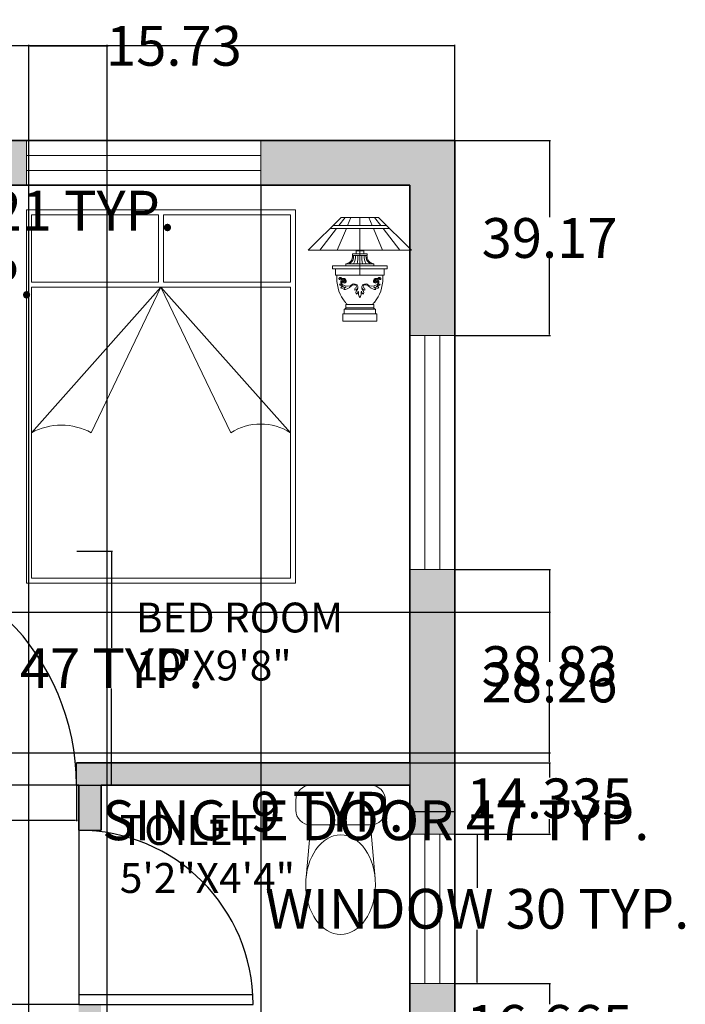
# Model space of a CAD drawing. Units: inches. Extents: x -24 to 368, y -370 to 58.
# Tile 9 of 9: x 235 to 368, y -140 to 58. Entities that reach past the tile are written whole.
import ezdxf

# ---------------------------------------------------------------- set-up
doc = ezdxf.new("R2010")
doc.units = ezdxf.units.IN
doc.header["$MEASUREMENT"] = 0
for name, color, linetype, lineweight in [('A-ANNO-DIMS', 2, 'Continuous', 18), ('A-AREA-IDEN', 7, 'Continuous', 18), ('A-FLOR-FIXT', 8, 'Continuous', 18), ('A-WALL', 7, 'Continuous', 35), ('Furniture', 7, 'Continuous', 15)]:
    doc.layers.add(name, color=color, linetype=linetype, lineweight=lineweight)
for name, color, linetype, lineweight, true_color in [('A-DOOR', 40, 'Continuous', 25, 0xf8d731), ('A-GLAZ', 30, 'Continuous', 18, 0xf26722), ('A-WALL-PATT', 18, 'Continuous', 13, 0x000000)]:
    doc.layers.add(name, color=color, linetype=linetype, lineweight=lineweight, true_color=true_color)
doc.styles.get("Standard").update_dxf_attribs({"font": 'arial.ttf'})
doc.dimstyles.get("Standard").update_dxf_attribs({"dimtxt": 8, "dimasz": 0.18, "dimexe": 0.18, "dimexo": 0.0625, "dimgap": 0.09, "dimtad": 0, "dimtih": 1, "dimtoh": 1, "dimdec": 4, "dimzin": 0, "dimdsep": 46, "dimlunit": 3, "dimtxsty": 'Standard', "dimcen": 0.09, "dimclre": 5, "dimclrt": 6, "dimadec": 0, "dimazin": 0, "dimtfac": 1, "dimtdec": 4, "dimtofl": 0, "dimtmove": 0, "dimatfit": 3, "dimfxl": 1, "dimtolj": 1, "dimtzin": 0, "dimarcsym": 0})

# ---------------------------------------------------------------- blocks, each defined once
blk = doc.blocks.new('LAMP-BEDSIDE')
for p, q in [((6.65, 20.8), (0, 14.26)), ((6.17, 19.19), (7.42, 20.8)), ((6.65, 20.8), (14.09, 20.8)), ((8.59, 20.8), (7.91, 19.19)), ((10.37, 20.8), (10.37, 19.19)), ((12.15, 20.8), (12.83, 19.19)), ((14.57, 19.19), (13.31, 20.8)), ((14.09, 20.8), (20.74, 14.26)), ((2.33, 14.26), (5.71, 18.6)), ((4.42, 18.6), (16.32, 18.6)), ((5.01, 19.19), (15.72, 19.19)), ((7.66, 18.6), (5.82, 14.26)), ((10.37, 18.6), (10.37, 9.21)), ((13.08, 18.6), (14.92, 14.26)), ((18.41, 14.26), (15.02, 18.6)), ((0, 14.26), (20.74, 14.26)), ((9.6, 14.09), (11.14, 14.09)), ((9.6, 14.09), (9.6, 13.52)), ((11.14, 14.09), (11.14, 13.52)), ((8.92, 13.52), (11.81, 13.52)), ((8.92, 13.52), (8.92, 13.19)), ((8.92, 13.19), (11.81, 13.19)), ((11.81, 13.52), (11.81, 13.19)), ((4.88, 11.13), (4.88, 10.49)), ((4.88, 11.13), (15.86, 11.13)), ((4.88, 10.49), (15.86, 10.49)), ((5.48, 10.49), (5.48, 9.21)), ((7.53, 11.52), (13.2, 11.52)), ((7.53, 11.52), (7.53, 11.13)), ((13.2, 11.52), (13.2, 11.13)), ((15.26, 10.49), (15.26, 9.21)), ((15.86, 11.13), (15.86, 10.49)), ((5.48, 9.21), (15.26, 9.21)), ((5.76, 9.21), (5.76, 8.59)), ((14.98, 9.21), (14.98, 8.59)), ((7.24, 2.43), (10.37, 2.43)), ((7.24, 2.43), (7.24, 1.48)), ((7.53, 3.34), (10.37, 3.34)), ((7.53, 3.34), (7.53, 2.65)), ((7.53, 2.65), (10.37, 2.65)), ((13.2, 3.34), (10.37, 3.34)), ((13.2, 2.65), (10.37, 2.65)), ((13.5, 2.43), (10.37, 2.43)), ((13.2, 3.34), (13.2, 2.65)), ((13.5, 2.43), (13.5, 1.48)), ((6.96, 1.48), (6.96, 0)), ((6.96, 1.48), (7.24, 1.48)), ((6.96, 0), (10.37, 0)), ((7.24, 1.48), (10.37, 1.48)), ((13.5, 1.48), (10.37, 1.48)), ((13.77, 0), (10.37, 0)), ((13.77, 1.48), (13.5, 1.48)), ((13.77, 1.48), (13.77, 0))]:
    blk.add_line(p, q)
for centre, radius, start, end in [((7.4, 13.04), 1.53, 274.9221, 5.4044), ((7.51, 13), 1.63, 295.0919, 6.6681), ((6.74, 12.97), 2.77, 328.5732, 4.5839), ((4.28, 12.92), 5.72, 345.8511, 2.7031), ((16.46, 12.92), 5.72, 177.2969, 194.1489), ((14, 12.97), 2.77, 175.4161, 211.4268), ((13.22, 13), 1.63, 173.3319, 244.9081), ((13.33, 13.04), 1.53, 174.5956, 265.0779), ((13.2, 8.5), 7.44, 179.3119, 219.4824), ((6.29, 8.51), 0.158, 124.9924, 335.335), ((6.45, 8.39), 0.355, 11.1092, 135.0155), ((6.39, 8.42), 0.0502, 145.048, 23.2806), ((6.51, 8.39), 0.171, 352.7452, 159.4145), ((7.39, 7.88), 0.87, 145.6908, 234.6789), ((7.4, 7.83), 0.668, 137.9008, 234.3868), ((7.12, 8.07), 0.5, 320.8911, 130.3323), ((7.11, 7.94), 0.236, 29.1955, 234.854), ((7.14, 8.08), 0.309, 326.7711, 139.3622), ((7.2, 8), 0.128, 26.7504, 223.4128), ((13.61, 8.07), 0.5, 49.6677, 219.1089), ((7.54, 8.5), 7.44, 320.5176, 0.6881), ((13.6, 8.08), 0.309, 40.6378, 213.2289), ((13.63, 7.94), 0.236, 305.146, 150.8045), ((13.54, 8), 0.128, 316.5872, 153.2496), ((13.34, 7.83), 0.668, 305.6132, 42.0992), ((13.34, 7.88), 0.87, 305.3211, 34.3092), ((14.29, 8.39), 0.355, 44.9845, 168.8908), ((14.23, 8.39), 0.171, 20.5855, 187.2548), ((14.45, 8.51), 0.158, 204.665, 55.0076), ((14.35, 8.42), 0.0502, 156.7194, 34.952), ((6.44, 6.9), 0.527, 30.7639, 106.5031), ((6.66, 7.53), 0.391, 199.4301, 258.0626), ((6.99, 6.45), 0.534, 81.7725, 150.3347), ((6.86, 7.15), 0.552, 231.7834, 300.6647), ((6.55, 6.3), 0.85, 53.0509, 88.4488), ((7.24, 8), 0.363, 223.4201, 318.9658), ((7.88, 8.48), 1.48, 232.7522, 313.7075), ((7.25, 8.05), 0.203, 224.103, 315.897), ((7.49, 6.32), 0.495, 75.8737, 133.8842), ((7.68, 6.3), 0.502, 98.3136, 177.606), ((7.04, 8.37), 2.05, 274.0547, 309.0162), ((5.53, 10.82), 4.92, 304.6293, 311.2979), ((9.22, 6.66), 0.644, 58.6818, 132.9572), ((9.12, 6.87), 0.587, 71.5671, 111.734), ((9.36, 6.81), 0.621, 342.0461, 94.8157), ((9.69, 6.38), 0.339, 108.5318, 204.8769), ((9.33, 6.92), 0.689, 273.9841, 333.6418), ((9.32, 6.94), 0.352, 316.7375, 49.0095), ((10.14, 5.79), 0.564, 138.2432, 224.6957), ((9.31, 6.66), 0.643, 310.3655, 356.3809), ((8.93, 6.11), 1.09, 318.697, 356.3018), ((9.3, 5.7), 0.788, 353.0671, 25.9825), ((11.43, 5.7), 0.788, 154.0175, 186.9329), ((11.81, 6.11), 1.09, 183.6982, 221.303), ((11.38, 6.81), 0.621, 85.1843, 197.9539), ((11.41, 6.92), 0.689, 206.3582, 266.0159), ((11.43, 6.66), 0.643, 183.6191, 229.6345), ((10.59, 5.79), 0.564, 315.3043, 41.7568), ((11.41, 6.94), 0.352, 130.9905, 223.2625), ((11.05, 6.38), 0.339, 335.1231, 71.4682), ((11.52, 6.66), 0.644, 47.0428, 121.3182), ((11.62, 6.87), 0.587, 68.266, 108.4329), ((12.85, 8.48), 1.48, 226.2925, 307.2478), ((15.2, 10.82), 4.92, 228.7021, 235.3707), ((13.7, 8.37), 2.05, 230.9838, 265.9453), ((13.25, 6.32), 0.495, 46.1158, 104.1263), ((13.05, 6.3), 0.502, 2.394, 81.6864), ((13.5, 8), 0.363, 221.0342, 316.5799), ((13.48, 8.05), 0.203, 224.103, 315.897), ((13.87, 7.15), 0.552, 239.3353, 308.2166), ((14.18, 6.3), 0.85, 91.5512, 126.9491), ((13.75, 6.45), 0.534, 29.6653, 98.2275), ((14.3, 6.9), 0.527, 73.4969, 149.2361), ((14.08, 7.53), 0.391, 281.9374, 340.5699), ((12.16, 5.83), 2.09, 186.3334, 210.8958), ((8.58, 5.83), 2.09, 329.1042, 353.6666), ((7.29, 2.67), 0.245, 257.4164, 350.592), ((10.43, 6.05), 3.74, 217.4462, 226.2556), ((10.31, 6.05), 3.74, 313.7444, 322.5538), ((10.31, 6.05), 3.74, 313.7444, 322.5538), ((13.45, 2.67), 0.245, 189.408, 282.5836)]:
    blk.add_arc(centre, radius, start, end)
blk = doc.blocks.new('WINDOW-47-JAMB-DETAIL')
for p, q in [((0, 9), (47, 9)), ((0, 0), (0, 9)), ((0, 9), (0, 4.5)), ((47, 9), (47, 0)), ((0, 6), (47, 6)), ((0, 3), (47, 3)), ((47, 0), (0, 0))]:
    blk.add_line(p, q)
blk = doc.blocks.new('WINDOW-47')
for p, q in [((0, 47), (0, 0)), ((0, 47), (9, 47)), ((3, 47), (3, 0)), ((6, 47), (6, 0)), ((9, 0), (9, 47)), ((0, 0), (9, 0))]:
    blk.add_line(p, q)
blk = doc.blocks.new('WINDOW-30')
for p, q in [((0, 9), (30, 9)), ((0, 0), (0, 9)), ((30, 9), (30, 0)), ((0, 6), (30, 6)), ((0, 3), (30, 3)), ((30, 0), (0, 0))]:
    blk.add_line(p, q)
blk = doc.blocks.new('DOOR-SINGLE-35')
for p, q in [((0, 35), (0, 0)), ((0, 35), (4.5, 35)), ((0, 2), (35, 2)), ((0, 0), (35, 0)), ((0, 0), (4.5, 0))]:
    blk.add_line(p, q)
blk.add_arc((0, 0), 35, 0, 90)
blk = doc.blocks.new('DOOR-SINGLE-47')
for p, q in [((0, 0), (0, 47)), ((2, 0), (2, 47)), ((47, 0), (0, 0))]:
    blk.add_line(p, q)
blk.add_arc((0, 0), 47, 0, 90)
blk = doc.blocks.new('*D13')
at = {"layer": 'A-ANNO-DIMS', "color": 5, "lineweight": -2, "transparency": 16777216}
for p, q in [((206.97, 16.43), (203.73, 16.43)), ((206.97, -4.37), (203.73, -4.37))]:
    blk.add_line(p, q, dxfattribs=at)
at = {"layer": 'A-ANNO-DIMS', "color": 0, "lineweight": -2, "transparency": 16777216}
for p, q in [((203.91, 16.25), (203.91, 10.14)), ((203.91, -4.19), (203.91, 1.92))]:
    blk.add_line(p, q, dxfattribs=at)
at = {"layer": 'A-ANNO-DIMS', "color": 0, "transparency": 16777216}
for points in [[(203.88, 16.25), (203.94, 16.25), (203.91, 16.43)], [(203.88, -4.19), (203.94, -4.19), (203.91, -4.37)]]:
    blk.add_solid(points, dxfattribs=at)
at = {"layer": 'Defpoints', "color": 0, "transparency": 16777216}
for p in [(203.91, 16.43), (207.03, 16.43), (207.03, -4.37)]:
    blk.add_point(p, dxfattribs=at)
at = {"layer": 'A-ANNO-DIMS', "color": 6, "transparency": 16777216, "insert": (203.91, 6.03), "char_height": 8, "attachment_point": 5}
blk.add_mtext('\\A1;LAMP 21 TYP.', dxfattribs=at)
blk = doc.blocks.new('*D14')
at = {"layer": 'A-ANNO-DIMS', "color": 5, "lineweight": -2, "transparency": 16777216}
for p, q in [((207.03, 16.49), (207.03, 19.73)), ((227.77, 16.49), (227.77, 19.73))]:
    blk.add_line(p, q, dxfattribs=at)
at = {"layer": 'A-ANNO-DIMS', "color": 0, "lineweight": -2, "transparency": 16777216}
for p, q in [((207.21, 19.55), (227.59, 19.55)), ((227.77, 19.55), (227.95, 19.55))]:
    blk.add_line(p, q, dxfattribs=at)
at = {"layer": 'A-ANNO-DIMS', "color": 0, "transparency": 16777216}
for points in [[(207.21, 19.58), (207.21, 19.52), (207.03, 19.55)], [(227.59, 19.58), (227.59, 19.52), (227.77, 19.55)]]:
    blk.add_solid(points, dxfattribs=at)
at = {"layer": 'Defpoints', "color": 0, "transparency": 16777216}
for p in [(227.77, 19.55), (207.03, 16.43), (227.77, 16.43)]:
    blk.add_point(p, dxfattribs=at)
at = {"layer": 'A-ANNO-DIMS', "color": 6, "transparency": 16777216, "insert": (247.58, 19.55), "char_height": 8, "attachment_point": 5}
blk.add_mtext('\\A1;21 TYP.', dxfattribs=at)
blk = doc.blocks.new('*D19')
at = {"layer": 'A-ANNO-DIMS', "color": 5, "lineweight": -2, "transparency": 16777216}
for p, q in [((199.21, -95.92), (199.21, -103.09)), ((246.21, -95.92), (246.21, -103.09))]:
    blk.add_line(p, q, dxfattribs=at)
at = {"layer": 'A-ANNO-DIMS', "color": 0, "lineweight": -2, "transparency": 16777216}
for p, q in [((199.39, -102.91), (246.03, -102.91)), ((246.21, -102.91), (246.39, -102.91))]:
    blk.add_line(p, q, dxfattribs=at)
at = {"layer": 'A-ANNO-DIMS', "color": 0, "transparency": 16777216}
for points in [[(199.39, -102.88), (199.39, -102.94), (199.21, -102.91)], [(246.03, -102.88), (246.03, -102.94), (246.21, -102.91)]]:
    blk.add_solid(points, dxfattribs=at)
at = {"layer": 'Defpoints', "color": 0, "transparency": 16777216}
for p in [(199.21, -95.86), (246.21, -95.86), (246.21, -102.91)]:
    blk.add_point(p, dxfattribs=at)
at = {"layer": 'A-ANNO-DIMS', "color": 6, "transparency": 16777216, "insert": (306.3, -102.91), "char_height": 8, "attachment_point": 5}
blk.add_mtext('\\A1;SINGLE DOOR 47 TYP.', dxfattribs=at)
blk = doc.blocks.new('*D20')
at = {"layer": 'A-ANNO-DIMS', "color": 5, "lineweight": -2, "transparency": 16777216}
for p, q in [((246.28, -48.86), (253.44, -48.86)), ((246.28, -95.86), (253.44, -95.86))]:
    blk.add_line(p, q, dxfattribs=at)
at = {"layer": 'A-ANNO-DIMS', "color": 0, "lineweight": -2, "transparency": 16777216}
for p, q in [((253.26, -49.04), (253.26, -68.26)), ((253.26, -95.68), (253.26, -76.45))]:
    blk.add_line(p, q, dxfattribs=at)
at = {"layer": 'A-ANNO-DIMS', "color": 0, "transparency": 16777216}
for points in [[(253.23, -49.04), (253.29, -49.04), (253.26, -48.86)], [(253.23, -95.68), (253.29, -95.68), (253.26, -95.86)]]:
    blk.add_solid(points, dxfattribs=at)
at = {"layer": 'Defpoints', "color": 0, "transparency": 16777216}
for p in [(246.21, -48.86), (253.26, -48.86), (246.21, -95.86)]:
    blk.add_point(p, dxfattribs=at)
at = {"layer": 'A-ANNO-DIMS', "color": 6, "transparency": 16777216, "insert": (253.26, -72.36), "char_height": 8, "attachment_point": 5}
blk.add_mtext('\\A1;47 TYP.', dxfattribs=at)
blk = doc.blocks.new('*D21')
at = {"layer": 'A-ANNO-DIMS', "color": 5, "lineweight": -2, "transparency": 16777216}
for p, q in [((322.22, -105.69), (326.84, -105.69)), ((322.22, -135.69), (326.84, -135.69))]:
    blk.add_line(p, q, dxfattribs=at)
at = {"layer": 'A-ANNO-DIMS', "color": 0, "lineweight": -2, "transparency": 16777216}
for p, q in [((326.66, -105.87), (326.66, -116.46)), ((326.66, -135.51), (326.66, -124.92))]:
    blk.add_line(p, q, dxfattribs=at)
at = {"layer": 'A-ANNO-DIMS', "color": 0, "transparency": 16777216}
for points in [[(326.63, -105.87), (326.69, -105.87), (326.66, -105.69)], [(326.63, -135.51), (326.69, -135.51), (326.66, -135.69)]]:
    blk.add_solid(points, dxfattribs=at)
at = {"layer": 'Defpoints', "color": 0, "transparency": 16777216}
for p in [(322.16, -105.69), (326.66, -105.69), (322.16, -135.69)]:
    blk.add_point(p, dxfattribs=at)
at = {"layer": 'A-ANNO-DIMS', "color": 6, "transparency": 16777216, "insert": (326.66, -120.69), "char_height": 8, "attachment_point": 5}
blk.add_mtext('\\A1;WINDOW 30 TYP.', dxfattribs=at)
blk = doc.blocks.new('*D22')
at = {"layer": 'A-ANNO-DIMS', "color": 0, "lineweight": -2, "transparency": 16777216}
for p, q in [((313.16, -101.19), (312.98, -101.19)), ((321.98, -101.19), (313.34, -101.19))]:
    blk.add_line(p, q, dxfattribs=at)
at = {"layer": 'A-ANNO-DIMS', "color": 5, "lineweight": -2, "transparency": 16777216}
for p, q in [((313.16, -105.63), (313.16, -101.01)), ((322.16, -105.63), (322.16, -101.01))]:
    blk.add_line(p, q, dxfattribs=at)
at = {"layer": 'A-ANNO-DIMS', "color": 0, "transparency": 16777216}
for points in [[(313.34, -101.16), (313.34, -101.22), (313.16, -101.19)], [(321.98, -101.16), (321.98, -101.22), (322.16, -101.19)]]:
    blk.add_solid(points, dxfattribs=at)
at = {"layer": 'Defpoints', "color": 0, "transparency": 16777216}
for p in [(313.16, -101.19), (313.16, -105.69), (322.16, -105.69)]:
    blk.add_point(p, dxfattribs=at)
at = {"layer": 'A-ANNO-DIMS', "color": 6, "transparency": 16777216, "insert": (296.53, -101.19), "char_height": 8, "attachment_point": 5}
blk.add_mtext('\\A1;9 TYP.', dxfattribs=at)
blk = doc.blocks.new('*D25')
at = {"layer": 'A-ANNO-DIMS', "color": 5, "lineweight": -2, "transparency": 16777216}
for p, q in [((4.16, 33.71), (4.16, 52.85)), ((322.16, 33.71), (322.16, 52.85))]:
    blk.add_line(p, q, dxfattribs=at)
at = {"layer": 'A-ANNO-DIMS', "color": 0, "lineweight": -2, "transparency": 16777216}
for p, q in [((4.34, 52.67), (154.23, 52.67)), ((321.98, 52.67), (172.1, 52.67))]:
    blk.add_line(p, q, dxfattribs=at)
at = {"layer": 'A-ANNO-DIMS', "color": 0, "transparency": 16777216}
for points in [[(4.34, 52.7), (4.34, 52.64), (4.16, 52.67)], [(321.98, 52.7), (321.98, 52.64), (322.16, 52.67)]]:
    blk.add_solid(points, dxfattribs=at)
at = {"layer": 'Defpoints', "color": 0, "transparency": 16777216}
for p in [(322.16, 52.67), (4.16, 33.64), (322.16, 33.64)]:
    blk.add_point(p, dxfattribs=at)
at = {"layer": 'A-ANNO-DIMS', "color": 6, "transparency": 16777216, "insert": (163.16, 52.67), "char_height": 8, "attachment_point": 5}
blk.add_mtext('\\A1;318', dxfattribs=at)
blk = doc.blocks.new('*D36')
at = {"layer": 'A-ANNO-DIMS', "color": 5, "lineweight": -2, "transparency": 16777216}
for p, q in [((322.22, -135.69), (341.36, -135.69)), ((313.22, -152.36), (341.36, -152.36))]:
    blk.add_line(p, q, dxfattribs=at)
at = {"layer": 'A-ANNO-DIMS', "color": 0, "lineweight": -2, "transparency": 16777216}
for p, q in [((341.18, -135.87), (341.18, -139.85)), ((341.18, -152.18), (341.18, -148.2))]:
    blk.add_line(p, q, dxfattribs=at)
at = {"layer": 'A-ANNO-DIMS', "color": 0, "transparency": 16777216}
for points in [[(341.15, -135.87), (341.21, -135.87), (341.18, -135.69)], [(341.15, -152.18), (341.21, -152.18), (341.18, -152.36)]]:
    blk.add_solid(points, dxfattribs=at)
at = {"layer": 'Defpoints', "color": 0, "transparency": 16777216}
for p in [(322.16, -135.69), (341.18, -135.69), (313.16, -152.36)]:
    blk.add_point(p, dxfattribs=at)
at = {"layer": 'A-ANNO-DIMS', "color": 6, "transparency": 16777216, "insert": (341.18, -144.02), "char_height": 8, "attachment_point": 5}
blk.add_mtext('\\A1;16.665', dxfattribs=at)
blk = doc.blocks.new('*D37')
at = {"layer": 'A-ANNO-DIMS', "color": 5, "lineweight": -2, "transparency": 16777216}
for p, q in [((313.22, -91.36), (341.36, -91.36)), ((322.22, -105.69), (341.36, -105.69))]:
    blk.add_line(p, q, dxfattribs=at)
at = {"layer": 'A-ANNO-DIMS', "color": 0, "lineweight": -2, "transparency": 16777216}
for p, q in [((341.18, -91.54), (341.18, -94.35)), ((341.18, -105.51), (341.18, -102.7))]:
    blk.add_line(p, q, dxfattribs=at)
at = {"layer": 'A-ANNO-DIMS', "color": 0, "transparency": 16777216}
for points in [[(341.15, -91.54), (341.21, -91.54), (341.18, -91.36)], [(341.15, -105.51), (341.21, -105.51), (341.18, -105.69)]]:
    blk.add_solid(points, dxfattribs=at)
at = {"layer": 'Defpoints', "color": 0, "transparency": 16777216}
for p in [(313.16, -91.36), (341.18, -91.36), (322.16, -105.69)]:
    blk.add_point(p, dxfattribs=at)
at = {"layer": 'A-ANNO-DIMS', "color": 6, "transparency": 16777216, "insert": (341.18, -98.52), "char_height": 8, "attachment_point": 5}
blk.add_mtext('\\A1;14.335', dxfattribs=at)
blk = doc.blocks.new('*D38')
at = {"layer": 'A-ANNO-DIMS', "color": 5, "lineweight": -2, "transparency": 16777216}
for p, q in [((322.22, -52.53), (341.36, -52.53)), ((313.22, -91.36), (341.36, -91.36))]:
    blk.add_line(p, q, dxfattribs=at)
at = {"layer": 'A-ANNO-DIMS', "color": 0, "lineweight": -2, "transparency": 16777216}
for p, q in [((341.18, -52.71), (341.18, -67.77)), ((341.18, -91.18), (341.18, -76.12))]:
    blk.add_line(p, q, dxfattribs=at)
at = {"layer": 'A-ANNO-DIMS', "color": 0, "transparency": 16777216}
for points in [[(341.15, -52.71), (341.21, -52.71), (341.18, -52.53)], [(341.15, -91.18), (341.21, -91.18), (341.18, -91.36)]]:
    blk.add_solid(points, dxfattribs=at)
at = {"layer": 'Defpoints', "color": 0, "transparency": 16777216}
for p in [(322.16, -52.53), (341.18, -52.53), (313.16, -91.36)]:
    blk.add_point(p, dxfattribs=at)
at = {"layer": 'A-ANNO-DIMS', "color": 6, "transparency": 16777216, "insert": (341.18, -71.94), "char_height": 8, "attachment_point": 5}
blk.add_mtext('\\A1;38.83', dxfattribs=at)
blk = doc.blocks.new('*D39')
at = {"layer": 'A-ANNO-DIMS', "color": 5, "lineweight": -2, "transparency": 16777216}
for p, q in [((322.22, 33.64), (341.36, 33.64)), ((322.22, -5.53), (341.36, -5.53))]:
    blk.add_line(p, q, dxfattribs=at)
at = {"layer": 'A-ANNO-DIMS', "color": 0, "lineweight": -2, "transparency": 16777216}
for p, q in [((341.18, 33.46), (341.18, 18.23)), ((341.18, -5.35), (341.18, 9.88))]:
    blk.add_line(p, q, dxfattribs=at)
at = {"layer": 'A-ANNO-DIMS', "color": 0, "transparency": 16777216}
for points in [[(341.15, 33.46), (341.21, 33.46), (341.18, 33.64)], [(341.15, -5.35), (341.21, -5.35), (341.18, -5.53)]]:
    blk.add_solid(points, dxfattribs=at)
at = {"layer": 'Defpoints', "color": 0, "transparency": 16777216}
for p in [(322.16, 33.64), (341.18, 33.64), (322.16, -5.53)]:
    blk.add_point(p, dxfattribs=at)
at = {"layer": 'A-ANNO-DIMS', "color": 6, "transparency": 16777216, "insert": (341.18, 14.06), "char_height": 8, "attachment_point": 5}
blk.add_mtext('\\A1;39.17', dxfattribs=at)
blk = doc.blocks.new('*D43')
at = {"layer": 'A-ANNO-DIMS', "color": 5, "lineweight": -2, "transparency": 16777216}
for p, q in [((283.21, 24.58), (283.21, -363.55)), ((313.16, 24.58), (313.16, -363.55))]:
    blk.add_line(p, q, dxfattribs=at)
at = {"layer": 'A-ANNO-DIMS', "color": 0, "lineweight": -2, "transparency": 16777216}
for p, q in [((283.39, -363.37), (284.5, -363.37)), ((312.98, -363.37), (311.87, -363.37))]:
    blk.add_line(p, q, dxfattribs=at)
at = {"layer": 'A-ANNO-DIMS', "color": 0, "transparency": 16777216}
for points in [[(283.39, -363.34), (283.39, -363.4), (283.21, -363.37)], [(312.98, -363.34), (312.98, -363.4), (313.16, -363.37)]]:
    blk.add_solid(points, dxfattribs=at)
at = {"layer": 'Defpoints', "color": 0, "transparency": 16777216}
for p in [(283.21, 24.64), (313.16, 24.64), (313.16, -363.37)]:
    blk.add_point(p, dxfattribs=at)
at = {"layer": 'A-ANNO-DIMS', "color": 6, "transparency": 16777216, "insert": (298.19, -363.37), "char_height": 8, "attachment_point": 5}
blk.add_mtext('\\A1;29.95', dxfattribs=at)
blk = doc.blocks.new('*D44')
at = {"layer": 'A-ANNO-DIMS', "color": 5, "lineweight": -2, "transparency": 16777216}
for p, q in [((13.22, -61.1), (341.36, -61.1)), ((13.22, -89.36), (341.36, -89.36))]:
    blk.add_line(p, q, dxfattribs=at)
at = {"layer": 'A-ANNO-DIMS', "color": 0, "lineweight": -2, "transparency": 16777216}
for p, q in [((341.18, -61.28), (341.18, -71.05)), ((341.18, -89.18), (341.18, -79.4))]:
    blk.add_line(p, q, dxfattribs=at)
at = {"layer": 'A-ANNO-DIMS', "color": 0, "transparency": 16777216}
for points in [[(341.15, -61.28), (341.21, -61.28), (341.18, -61.1)], [(341.15, -89.18), (341.21, -89.18), (341.18, -89.36)]]:
    blk.add_solid(points, dxfattribs=at)
at = {"layer": 'Defpoints', "color": 0, "transparency": 16777216}
for p in [(13.16, -61.1), (341.18, -61.1), (13.16, -89.36)]:
    blk.add_point(p, dxfattribs=at)
at = {"layer": 'A-ANNO-DIMS', "color": 6, "transparency": 16777216, "insert": (341.18, -75.23), "char_height": 8, "attachment_point": 5}
blk.add_mtext('\\A1;28.26', dxfattribs=at)
blk = doc.blocks.new('*D59')
at = {"layer": 'A-ANNO-DIMS', "color": 5, "lineweight": -2, "transparency": 16777216}
for p, q in [((246.6, -139.91), (-15.03, -139.91)), ((246.6, -147.86), (-15.03, -147.86))]:
    blk.add_line(p, q, dxfattribs=at)
at = {"layer": 'A-ANNO-DIMS', "color": 0, "lineweight": -2, "transparency": 16777216}
for p, q in [((-14.85, -139.91), (-14.85, -139.73)), ((-14.85, -139.73), (-14.67, -139.73)), ((-14.85, -147.68), (-14.85, -140.09))]:
    blk.add_line(p, q, dxfattribs=at)
at = {"layer": 'A-ANNO-DIMS', "color": 0, "transparency": 16777216}
for points in [[(-14.88, -140.09), (-14.82, -140.09), (-14.85, -139.91)], [(-14.88, -147.68), (-14.82, -147.68), (-14.85, -147.86)]]:
    blk.add_solid(points, dxfattribs=at)
at = {"layer": 'Defpoints', "color": 0, "transparency": 16777216}
for p in [(-14.85, -139.91), (246.66, -139.91), (246.66, -147.86)]:
    blk.add_point(p, dxfattribs=at)
at = {"layer": 'A-ANNO-DIMS', "color": 6, "transparency": 16777216, "insert": (-4.2, -139.73), "char_height": 8, "attachment_point": 5}
blk.add_mtext('\\A1;7.95', dxfattribs=at)
blk = doc.blocks.new('*D61')
at = {"layer": 'A-ANNO-DIMS', "color": 5, "lineweight": -2, "transparency": 16777216}
for p, q in [((236.66, -275.29), (236.66, 52.85)), ((252.39, -275.29), (252.39, 52.85))]:
    blk.add_line(p, q, dxfattribs=at)
at = {"layer": 'A-ANNO-DIMS', "color": 0, "lineweight": -2, "transparency": 16777216}
for p, q in [((236.84, 52.67), (252.21, 52.67)), ((252.39, 52.67), (252.57, 52.67))]:
    blk.add_line(p, q, dxfattribs=at)
at = {"layer": 'A-ANNO-DIMS', "color": 0, "transparency": 16777216}
for points in [[(236.84, 52.7), (236.84, 52.64), (236.66, 52.67)], [(252.21, 52.7), (252.21, 52.64), (252.39, 52.67)]]:
    blk.add_solid(points, dxfattribs=at)
at = {"layer": 'Defpoints', "color": 0, "transparency": 16777216}
for p in [(252.39, 52.67), (236.66, -275.36), (252.39, -275.36)]:
    blk.add_point(p, dxfattribs=at)
at = {"layer": 'A-ANNO-DIMS', "color": 6, "transparency": 16777216, "insert": (265.78, 52.67), "char_height": 8, "attachment_point": 5}
blk.add_mtext('\\A1;15.73', dxfattribs=at)

msp = doc.modelspace()

# ---------------------------------------------------------------- hatches: boundary and pattern name
at = {"layer": 'A-WALL-PATT'}
h = msp.add_hatch(color=256, dxfattribs=at)
h.dxf.hatch_style = 1
h.paths.add_polyline_path([(13.1621, -93.8573), (80.4499, -93.8573), (80.4499, -89.3573), (13.1621, -89.3573), (13.1621, -61.0987), (4.1621, -61.0987), (4.1621, -149.8573), (13.1621, -149.8573)])
h.paths.add_polyline_path([(146.5668, -27.3573), (133.1621, -27.3573), (133.1621, 10.3323), (133.1272, 10.3313), (133.1621, 24.6427), (139.8141, 24.6427), (139.8141, 33.6427), (95.3329, 33.6427), (95.3329, 24.6427), (128.6621, 24.6427), (128.6621, -89.3573), (127.4499, -89.3573), (127.4499, -93.8573), (133.1621, -93.8573), (133.1621, -31.8573), (146.5668, -31.8573)])
h.paths.add_polyline_path([(197.6621, 24.6427), (236.2134, 24.6427), (236.2134, 33.6427), (169.8141, 33.6427), (169.8141, 24.6427), (193.1621, 24.6427), (193.1621, -27.3573), (181.5668, -27.3573), (181.5668, -31.8573), (193.1621, -31.8573), (193.1621, -95.8573), (199.2127, -95.8573), (199.2127, -91.3573), (197.6621, -91.3573)])
h.paths.add_polyline_path([(322.1621, -52.531), (313.1621, -52.531), (313.1621, -91.3573), (246.2127, -91.3573), (246.2127, -95.8573), (246.6621, -95.8573), (246.6621, -104.9077), (251.1621, -104.9077), (251.1621, -95.8573), (313.1621, -95.8573), (313.1621, -105.6922), (317.6621, -105.6922), (322.1621, -105.6922)])
h.paths.add_polyline_path([(322.1621, -135.6922), (313.1621, -135.6922), (313.1621, -147.8573), (251.1621, -147.8573), (251.1621, -139.9077), (246.6621, -139.9077), (246.6621, -147.8573), (199.43, -147.8573), (199.43, -152.3573), (313.1621, -152.3573), (313.1621, -194.6142), (317.6621, -194.6142), (322.1621, -194.6142)])
h.paths.add_polyline_path([(322.1621, -241.6142), (313.1621, -241.6142), (313.1621, -275.3573), (287.3912, -275.3573), (287.3912, -279.8573), (313.1621, -279.8573), (313.1621, -335.3573), (298.077, -335.3573), (298.077, -344.3573), (322.1621, -344.3573)])
h.paths.add_polyline_path([(263.077, -335.3573), (241.1621, -335.3573), (241.1621, -279.8573), (252.3912, -279.8573), (252.3912, -275.3573), (236.6621, -275.3573), (236.6621, -298.8573), (234.5689, -298.8573), (234.5689, -303.3573), (236.6621, -303.3573), (236.6621, -344.3573), (263.077, -344.3573), (263.077, -339.8573)])
h.paths.add_polyline_path([(175.5689, -298.8573), (131.6621, -298.8573), (131.6621, -152.3573), (164.43, -152.3573), (164.43, -147.8573), (127.1621, -147.8573), (127.1621, -232.8573), (117.1621, -232.8573), (117.1621, -237.3573), (127.1621, -237.3573), (127.1621, -335.3573), (84.4055, -335.3573), (84.4055, -344.3573), (131.6621, -344.3573), (131.6621, -303.3573), (175.5689, -303.3573)])
h.paths.add_polyline_path([(70.1621, -232.8573), (13.1621, -232.8573), (13.1621, -196.8573), (4.1621, -196.8573), (4.1621, -257.9061), (13.1621, -257.9061), (13.1621, -237.3573), (70.1621, -237.3573)])
h.paths.add_polyline_path([(13.1621, -304.9061), (4.1621, -304.9061), (4.1621, -344.3573), (37.4055, -344.3573), (37.4055, -335.3573), (13.1621, -335.3573)])
h.paths.add_polyline_path([(322.1621, 33.6427), (283.2134, 33.6427), (283.2134, 24.6427), (313.1621, 24.6427), (313.1621, 11.9273), (313.4656, 11.629), (313.1621, 11.629), (313.1621, -5.531), (322.1621, -5.531)])
h.paths.add_polyline_path([(48.3329, 33.6427), (4.1621, 33.6427), (4.1621, -14.0987), (13.1621, -14.0987), (13.1621, 24.6427), (48.3329, 24.6427)])

# ---------------------------------------------------------------- linework, layer by layer
at = {"layer": 'A-DOOR'}
msp.add_line((246.2127, -95.8573), (246.2127, -91.3573), dxfattribs=at)
at = {"layer": 'A-FLOR-FIXT'}
for p, q in [((293.2418, -95.8573), (305.2418, -95.8573)), ((290.2418, -100.8573), (290.2418, -98.8573)), ((308.2418, -98.8573), (308.2418, -100.8573)), ((293.2418, -103.8573), (292.3192, -114.3746)), ((305.2418, -103.8573), (293.2418, -103.8573)), ((305.2418, -103.8573), (306.1872, -114.6112))]:
    msp.add_line(p, q, dxfattribs=at)
for centre, start, end in [((293.2418, -98.8573), 90, 180), ((305.2418, -98.8573), 0, 90), ((293.2418, -100.8573), 180, 270), ((305.2418, -100.8573), 270, 0)]:
    msp.add_arc(centre, 3, start, end, dxfattribs=at)
msp.add_ellipse((299.2418, -115.8573), major_axis=(0, -10), ratio=0.7, dxfattribs=at)
at = {"layer": 'A-GLAZ'}
msp.add_line((313.1621, -105.6922), (317.6621, -105.6922), dxfattribs=at)
at = {"layer": 'A-WALL'}
for p, q in [((4.1621, 33.6427), (322.1621, 33.6427)), ((322.1621, 33.6427), (322.1621, -344.3573)), ((197.6621, 24.6427), (313.1621, 24.6427)), ((313.1621, 24.6427), (313.1621, -91.3573)), ((246.2127, -91.3573), (313.1621, -91.3573)), ((246.2127, -95.8573), (246.6621, -95.8573)), ((246.6621, -95.8573), (246.6621, -104.9077)), ((251.1621, -95.8573), (251.1621, -104.9077)), ((251.1621, -95.8573), (313.1621, -95.8573)), ((313.1621, -95.8573), (313.1621, -147.8573))]:
    msp.add_line(p, q, dxfattribs=at)
at = {"layer": 'Furniture'}
for p, q in [((262.6757, 5.1724), (262.6757, 18.7022)), ((263.6757, 5.1724), (263.6757, 18.7022)), ((237.1757, 5.1724), (262.6757, 5.1724)), ((237.1757, 4.1724), (289.1757, 4.1724)), ((263.1757, 4.1724), (237.1757, -25.0627)), ((249.1757, -25.0627), (263.1757, 4.1724)), ((263.1757, 4.1724), (289.1757, -25.0627)), ((277.1757, -25.0627), (263.1757, 4.1724)), ((263.6757, 5.1724), (289.1757, 5.1724))]:
    msp.add_line(p, q, dxfattribs=at)
msp.add_lwpolyline([(236.1757, 19.7022), (290.1757, 19.7022), (290.1757, -55.2978), (236.1757, -55.2978)], close=True, dxfattribs=at)
for points in [[(237.1757, 5.1724), (237.1757, 18.7022), (262.6757, 18.7022)], [(263.6757, 18.7022), (289.1757, 18.7022), (289.1757, 5.1724)], [(289.1757, 4.1724), (289.1757, -54.2978), (237.1757, -54.2978), (237.1757, 4.1724)]]:
    msp.add_lwpolyline(points, dxfattribs=at)
for centre, radius, start, end in [((243.1757, -36.0783), 12.5437, 61.423752, 118.576248), ((283.1757, -34.4581), 11.1478, 57.437311, 122.562689)]:
    msp.add_arc(centre, radius, start, end, dxfattribs=at)

# ---------------------------------------------------------------- block references
at = {"layer": 'A-DOOR'}
for name, p in [('DOOR-SINGLE-47', (199.213, -95.857)), ('DOOR-SINGLE-35', (246.662, -139.908))]:
    msp.add_blockref(name, p, dxfattribs=at)
at = {"layer": 'A-GLAZ'}
for name, p in [('WINDOW-47-JAMB-DETAIL', (236.213, 24.643)), ('WINDOW-47', (313.162, -52.5308))]:
    msp.add_blockref(name, p, dxfattribs=at)
at = {"layer": 'A-GLAZ', "rotation": 90.00000000000003}
msp.add_blockref('WINDOW-30', (322.1618, -135.6923), dxfattribs=at)
at = {"layer": 'Furniture'}
msp.add_blockref('LAMP-BEDSIDE', (292.73, -2.6353), dxfattribs=at)

# ---------------------------------------------------------------- texts
at = {"layer": 'A-AREA-IDEN'}
for s, p in [('BED ROOM', (258.1174, -65.1874)), ('10\'X9\'8"', (258.1174, -74.8259)), ('TOILET', (254.9137, -107.8684)), ('5\'2"X4\'4"', (254.9137, -117.5069))]:
    msp.add_text(s, height=6, dxfattribs=at).set_placement(p)

# ---------------------------------------------------------------- dimensions: what is measured, and where the dimension line sits
at = {"layer": 'A-ANNO-DIMS'}
for base, p1, p2, override, picture, middle in [((322.1621, 52.6658), (4.1621, 33.6427), (322.1621, 33.6427), {"dimdec": 0, "dimlfac": 1, "dimrnd": 0, "dimzin": 0, "dimdsep": 46, "dimlunit": 2}, '*D25', (163.1621, 52.6658)), ((252.3912, 52.6658), (236.6621, -275.3573), (252.3912, -275.3573), {"dimdec": 2, "dimlfac": 1, "dimrnd": 0, "dimzin": 0, "dimdsep": 46, "dimlunit": 2}, '*D61', (265.7827, 52.6658)), ((313.1621, -363.3723), (283.2134, 24.6427), (313.1621, 24.6427), {"dimdec": 2, "dimlfac": 1, "dimrnd": 0, "dimzin": 0, "dimdsep": 46, "dimlunit": 2}, '*D43', (298.1877, -363.3723))]:
    dim = msp.add_linear_dim(base=base, p1=p1, p2=p2, dimstyle='Standard', override=override, dxfattribs=at)
    dim.commit()
    dim.dimension.update_dxf_attribs({"geometry": picture, "text_midpoint": middle})
for base, p1, p2, override, picture, middle in [((341.1771, 33.6427), (322.1621, -5.531), (322.1621, 33.6427), {"dimdec": 2, "dimlfac": 1, "dimrnd": 0, "dimzin": 0, "dimdsep": 46, "dimlunit": 2}, '*D39', (341.1771, 14.0559)), ((341.1771, -52.531), (313.1621, -91.3573), (322.1621, -52.531), {"dimdec": 2, "dimlfac": 1, "dimrnd": 0, "dimzin": 0, "dimdsep": 46, "dimlunit": 2}, '*D38', (341.1771, -71.9441)), ((341.1771, -61.0987), (13.1621, -89.3573), (13.1621, -61.0987), {"dimdec": 2, "dimlfac": 1, "dimrnd": 0, "dimzin": 0, "dimdsep": 46, "dimlunit": 2}, '*D44', (341.1771, -75.228)), ((341.1771, -91.3573), (322.1621, -105.6922), (313.1621, -91.3573), {"dimdec": 3, "dimlfac": 1, "dimrnd": 0, "dimzin": 0, "dimdsep": 46, "dimlunit": 2}, '*D37', (341.1771, -98.5247)), ((-14.8529, -139.9077), (246.6621, -147.8573), (246.6621, -139.9077), {"dimdec": 2, "dimlfac": 1, "dimrnd": 0, "dimzin": 0, "dimdsep": 46, "dimlunit": 2}, '*D59', (-4.1955, -139.7277)), ((341.1771, -135.6922), (313.1621, -152.3573), (322.1621, -135.6922), {"dimdec": 3, "dimlfac": 1, "dimrnd": 0, "dimzin": 0, "dimdsep": 46, "dimlunit": 2}, '*D36', (341.1771, -144.0247))]:
    dim = msp.add_linear_dim(base=base, p1=p1, p2=p2, angle=90, dimstyle='Standard', override=override, dxfattribs=at)
    dim.commit()
    dim.dimension.update_dxf_attribs({"geometry": picture, "text_midpoint": middle})
for base, p1, p2, text, picture, middle in [((227.7689, 19.5455), (207.0338, 16.4258), (227.7689, 16.4258), '<> TYP.', '*D14', (247.5778, 19.5455)), ((246.2127, -102.9073), (199.2127, -95.8573), (246.2127, -95.8573), 'SINGLE DOOR <> TYP.', '*D19', (306.2999, -102.9073))]:
    dim = msp.add_linear_dim(base=base, p1=p1, p2=p2, text=text, dimstyle='Standard', override={"dimdec": 0, "dimlfac": 1, "dimrnd": 0, "dimzin": 0, "dimdsep": 46, "dimlunit": 2}, dxfattribs=at)
    dim.commit()
    dim.dimension.update_dxf_attribs({"geometry": picture, "text_midpoint": middle})
for base, p1, p2, angle, text, picture, middle in [((203.9141, 16.4258), (207.0338, -4.3721), (207.0338, 16.4258), 90, 'LAMP <> TYP.', '*D13', (203.9141, 6.0268)), ((253.2627, -48.8573), (246.2127, -95.8573), (246.2127, -48.8573), 90, '<> TYP.', '*D20', (253.2627, -72.3573)), ((313.1621, -101.1922), (322.1621, -105.6922), (313.1621, -105.6922), 180, '<> TYP.', '*D22', (296.5292, -101.1922)), ((326.6621, -105.6922), (322.1621, -135.6922), (322.1621, -105.6922), 90, 'WINDOW <> TYP.', '*D21', (326.6621, -120.6922))]:
    dim = msp.add_linear_dim(base=base, p1=p1, p2=p2, angle=angle, text=text, dimstyle='Standard', override={"dimdec": 0, "dimlfac": 1, "dimrnd": 0, "dimzin": 0, "dimdsep": 46, "dimlunit": 2}, dxfattribs=at)
    dim.commit()
    dim.dimension.update_dxf_attribs({"geometry": picture, "text_midpoint": middle})

doc.saveas('drawing.dxf')
